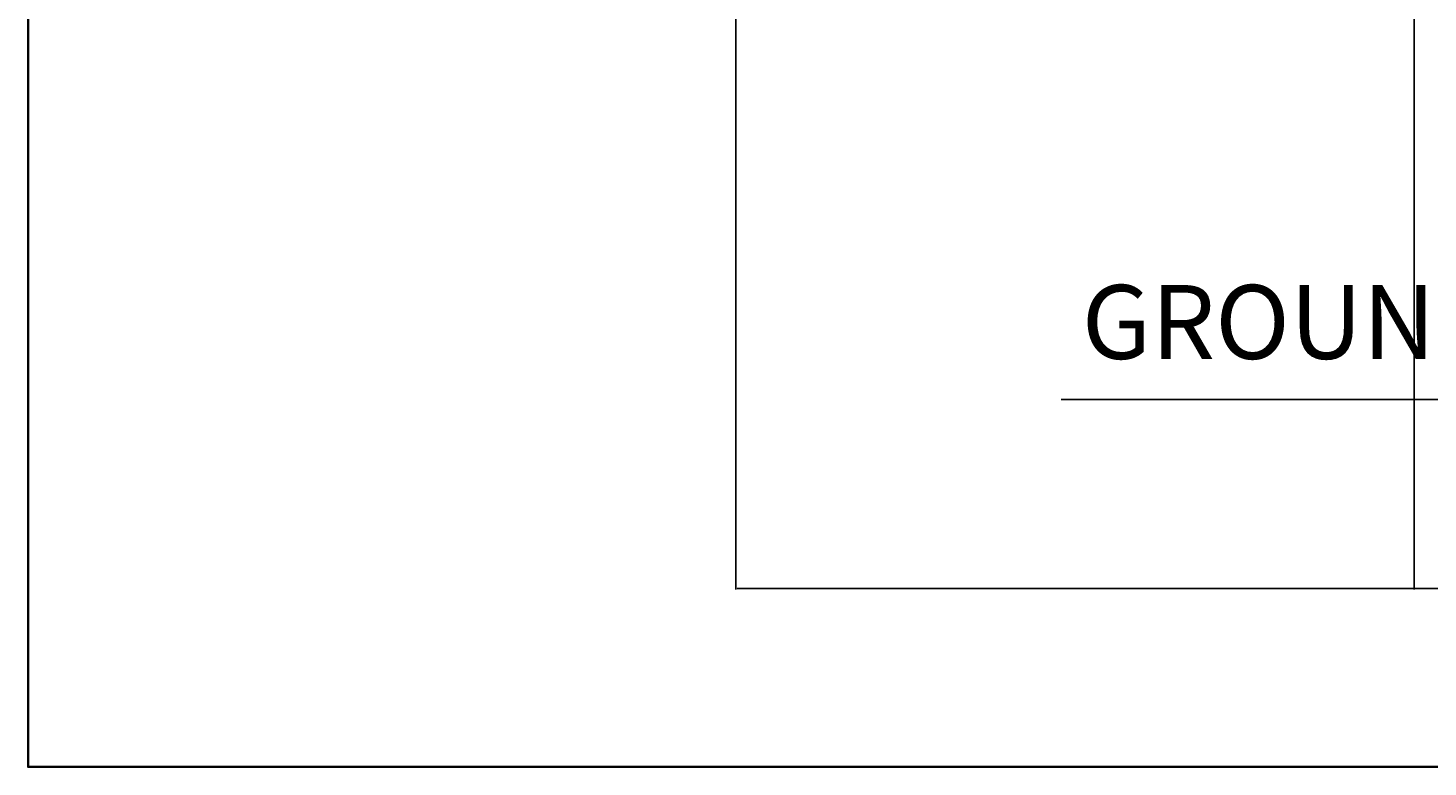
# Model space of a CAD drawing. Units: inches. Extents: x 1911 to 3278, y 2022 to 3108.
# Tile 1 of 13: x 1911 to 2120, y 2022 to 2132. Entities that reach past the tile are written whole.
import ezdxf

# ---------------------------------------------------------------- set-up
doc = ezdxf.new("R2010")
doc.units = ezdxf.units.IN
for name, color, linetype, lineweight in [('A-ANNO-DIMS', 2, 'Continuous', 18), ('A-ANNO-TITL', 7, 'Continuous', 25), ('A-ANNO-TTLB', 7, 'Continuous', 35)]:
    doc.layers.add(name, color=color, linetype=linetype, lineweight=lineweight)
doc.styles.get("Standard").update_dxf_attribs({"font": 'arial.ttf'})
doc.dimstyles.get("Standard").update_dxf_attribs({"dimtxt": 0.18, "dimasz": 0.18, "dimexe": 0.18, "dimexo": 0.0625, "dimgap": 0.09, "dimtad": 0, "dimtih": 1, "dimtoh": 1, "dimdec": 4, "dimzin": 0, "dimdsep": 46, "dimtxsty": 'Standard', "dimcen": 0.09, "dimadec": 0, "dimazin": 0, "dimtfac": 1, "dimtdec": 4, "dimtofl": 0, "dimtmove": 0, "dimatfit": 3, "dimfxl": 1, "dimtolj": 1, "dimtzin": 0, "dimarcsym": 0})

# ---------------------------------------------------------------- blocks, each defined once
blk = doc.blocks.new('*D68')
at = {"layer": 'A-ANNO-DIMS', "color": 0, "lineweight": -2, "transparency": 16777216}
for p, q in [((2016.83, 2263.81), (2016.83, 2048.12)), ((2117.83, 2263.81), (2117.83, 2048.12)), ((2017.01, 2048.3), (2067.07, 2048.3)), ((2117.65, 2048.3), (2067.6, 2048.3))]:
    blk.add_line(p, q, dxfattribs=at)
at = {"layer": 'A-ANNO-DIMS', "color": 0, "transparency": 16777216}
for points in [[(2017.01, 2048.33), (2017.01, 2048.27), (2016.83, 2048.3)], [(2117.65, 2048.33), (2117.65, 2048.27), (2117.83, 2048.3)]]:
    blk.add_solid(points, dxfattribs=at)
at = {"layer": 'Defpoints', "color": 0, "transparency": 16777216}
for p in [(2016.83, 2263.87), (2117.83, 2263.87), (2117.83, 2048.3)]:
    blk.add_point(p, dxfattribs=at)
at = {"layer": 'A-ANNO-DIMS', "color": 0, "transparency": 16777216, "insert": (2067.33, 2048.3), "char_height": 0.18, "attachment_point": 5}
blk.add_mtext('\\A1;101', dxfattribs=at)
blk = doc.blocks.new('*D70')
at = {"layer": 'A-ANNO-DIMS', "color": 0, "lineweight": -2, "transparency": 16777216}
for p, q in [((2134.1, 2181.81), (2134.1, 2048.12)), ((2016.83, 2133.81), (2016.83, 2048.12)), ((2017.01, 2048.3), (2075.01, 2048.3)), ((2133.92, 2048.3), (2075.92, 2048.3))]:
    blk.add_line(p, q, dxfattribs=at)
at = {"layer": 'A-ANNO-DIMS', "color": 0, "transparency": 16777216}
for points in [[(2017.01, 2048.33), (2017.01, 2048.27), (2016.83, 2048.3)], [(2133.92, 2048.33), (2133.92, 2048.27), (2134.1, 2048.3)]]:
    blk.add_solid(points, dxfattribs=at)
at = {"layer": 'Defpoints', "color": 0, "transparency": 16777216}
for p in [(2134.1, 2181.87), (2016.83, 2133.87), (2134.1, 2048.3)]:
    blk.add_point(p, dxfattribs=at)
at = {"layer": 'A-ANNO-DIMS', "color": 0, "transparency": 16777216, "insert": (2075.47, 2048.3), "char_height": 0.18, "attachment_point": 5}
blk.add_mtext('\\A1;117.27', dxfattribs=at)

msp = doc.modelspace()

# ---------------------------------------------------------------- linework, layer by layer
at = {"layer": 'A-ANNO-TITL'}
msp.add_line((2065.2731, 2076.4043), (2238.4413, 2076.4043), dxfattribs=at)
at = {"layer": 'A-ANNO-TTLB'}
msp.add_lwpolyline([(1911.3875, 3108.0628), (3278.3142, 3108.0628), (3278.3142, 2021.7237), (1911.3875, 2021.7237)], close=True, dxfattribs=at)

# ---------------------------------------------------------------- texts
at = {"layer": 'A-ANNO-TITL', "insert": (2068.3363, 2093.4469), "char_height": 11, "attachment_point": 1}
msp.add_mtext_dynamic_manual_height_columns('GROUND FLOOR PLAN', width=300.572415, gutter_width=12.5, heights=[0], dxfattribs=at)

# ---------------------------------------------------------------- dimensions: what is measured, and where the dimension line sits
at = {"layer": 'A-ANNO-DIMS'}
for base, p1, p2, override, picture, middle in [((2117.8344, 2048.3043), (2016.8344, 2263.8733), (2117.8344, 2263.8733), {"dimdec": 0, "dimlfac": 1, "dimrnd": 0, "dimzin": 0, "dimdsep": 46, "dimlunit": 2}, '*D68', (2067.3344, 2048.3043)), ((2134.1034, 2048.3043), (2016.8344, 2133.8733), (2134.1034, 2181.8733), {"dimdec": 2, "dimlfac": 1, "dimrnd": 0, "dimzin": 0, "dimdsep": 46, "dimlunit": 2}, '*D70', (2075.4689, 2048.3043))]:
    dim = msp.add_linear_dim(base=base, p1=p1, p2=p2, dimstyle='Standard', override=override, dxfattribs=at)
    dim.commit()
    dim.dimension.update_dxf_attribs({"geometry": picture, "text_midpoint": middle})

doc.saveas('drawing.dxf')
